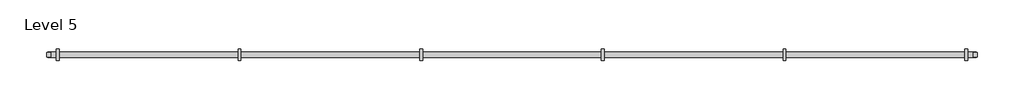
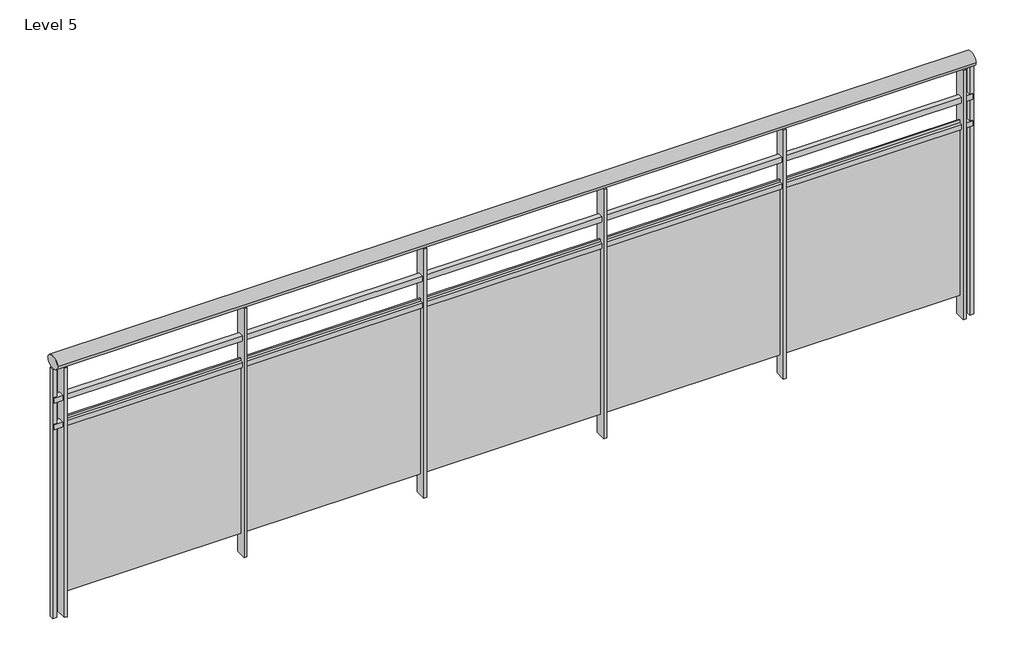
# One storey: 1 railing.
"""IFC4 building model written with IfcOpenShell, lengths in millimetres."""

from ifc_helpers import new_model, si_unit, point, frame, origin, place, context, project, spatial, polyline, ellipse_curve, trimmed, outline, extrude, element, save
from ifc_brep_helpers import plane_surface, extruded_surface, advanced_brep

model = new_model("IFC4")

# Units and contexts
model_context = context("Model", 3, world=origin())
ifc_project = project(units=[si_unit("LENGTHUNIT", "METRE", prefix="MILLI")], contexts=[model_context])

# Site, building, storey
site = spatial("IfcSite", under=ifc_project)
building = spatial("IfcBuilding", under=site)
storey = spatial("IfcBuildingStorey", under=building, Name="Level 5", Elevation=12801.6)

# Railing
placement = place(None, origin())
element("IfcRailing", 1, ObjectType="Glass Panel - Bottom Fill", at=placement, inside=storey, context=model_context, shape_type="SolidModel", body=[
    advanced_brep(
    [(-5729.1673724, -5829.5544725, 14020.8), (-5729.1673724, -5905.7544725, 14020.8), (-1576.8982041, -5829.5544725, 14020.8), (-1576.8982041, -5905.7544725, 14020.8)],
    [
        (0, 1, ellipse_curve(frame((-5729.1673724, -5867.6544725, 14020.8), z_axis=(-1.0, 0.0, 0.0), x_axis=(0.0, -1.0, 0.0)), 38.1, 28.575)),
        (1, 0, ellipse_curve(frame((-5729.1673724, -5867.6544725, 14020.8), z_axis=(-1.0, 0.0, 0.0), x_axis=(0.0, -1.0, 0.0)), 38.1, 28.575)),
        (2, 3, ellipse_curve(frame((-1576.8982041, -5867.6544725, 14020.8), z_axis=(1.0, 0.0, 0.0), x_axis=(0.0, -1.0, 0.0)), 38.1, 28.575)),
        (3, 2, ellipse_curve(frame((-1576.8982041, -5867.6544725, 14020.8), z_axis=(1.0, 0.0, 0.0), x_axis=(0.0, -1.0, 0.0)), 38.1, 28.575)),
        (0, 2),
        (3, 1),
    ],
    [
        plane_surface(frame((-5729.1673724, -5867.6544725, 14020.8), z_axis=(-1.0, 0.0, 0.0), x_axis=(0.0, 1.0, 0.0))),
        plane_surface(frame((-1576.8982041, -5867.6544725, 14020.8), z_axis=(1.0, 0.0, 0.0), x_axis=(0.0, 1.0, 0.0))),
        extruded_surface(trimmed(ellipse_curve(frame((-1576.8982041, -5867.6544725, 14020.8), z_axis=(-1.0, 0.0, 0.0), x_axis=(0.0, -1.0, 0.0)), 38.1, 28.575), [point((-1576.8982041, -5829.5544725, 14020.8))], [point((-1576.8982041, -5905.7544725, 14020.8))], True, "CARTESIAN"), (-4152.2691683, 0.0, 0.0), 4152.2691683),
        extruded_surface(trimmed(ellipse_curve(frame((-1576.8982041, -5867.6544725, 14020.8), z_axis=(-1.0, 0.0, 0.0), x_axis=(0.0, -1.0, 0.0)), 38.1, 28.575), [point((-1576.8982041, -5905.7544725, 14020.8))], [point((-1576.8982041, -5829.5544725, 14020.8))], True, "CARTESIAN"), (-4152.2691683, 0.0, 0.0), 4152.2691683),
    ],
    [
        (0, [[1, 2]]),
        (1, [[3, 4]]),
        (2, [[-1, 5, -4, 6]]),
        (3, [[-2, -6, -3, -5]]),
    ],
),
    extrude(outline(polyline([(-5729.1673724, -5880.3544725), (-5729.1673724, -5854.9544725), (-1576.8982041, -5854.9544725), (-1576.8982041, -5880.3544725), (-5729.1673724, -5880.3544725)])), frame((0.0, 0.0, 13830.3), z_axis=(0.0, 0.0, 1.0), x_axis=(1.0, 0.0, 0.0)), (0.0, 0.0, 1.0), 25.4),
    extrude(outline(polyline([(-5729.1673724, -5880.3544725), (-5729.1673724, -5854.9544725), (-1576.8982041, -5854.9544725), (-1576.8982041, -5880.3544725), (-5729.1673724, -5880.3544725)])), frame((0.0, 0.0, 13703.3), z_axis=(0.0, 0.0, 1.0), x_axis=(1.0, 0.0, 0.0)), (0.0, 0.0, 1.0), 25.4),
    extrude(outline(polyline([(-1627.3827882, -5893.0544725), (-1627.3827882, -5842.2544725), (-1614.6827882, -5842.2544725), (-1614.6827882, -5893.0544725), (-1627.3827882, -5893.0544725)])), frame((0.0, 0.0, 12801.6), z_axis=(0.0, 0.0, 1.0), x_axis=(1.0, 0.0, 0.0)), (0.0, 0.0, 1.0), 1190.625),
    extrude(outline(polyline([(-2433.8327882, -5861.1193155), (-1621.0327882, -5861.1193155), (-1621.0327882, -5867.4693155), (-2433.8327882, -5867.4693155), (-2433.8327882, -5861.1193155)])), frame((0.0, 0.0, 12903.2), z_axis=(0.0, 0.0, 1.0), x_axis=(1.0, 0.0, 0.0)), (0.0, 0.0, 1.0), 838.2),
    extrude(outline(polyline([(-2440.1827882, -5893.0544725), (-2440.1827882, -5842.2544725), (-2427.4827882, -5842.2544725), (-2427.4827882, -5893.0544725), (-2440.1827882, -5893.0544725)])), frame((0.0, 0.0, 12801.6), z_axis=(0.0, 0.0, 1.0), x_axis=(1.0, 0.0, 0.0)), (0.0, 0.0, 1.0), 1190.625),
    extrude(outline(polyline([(-3246.6327882, -5861.1193155), (-2433.8327882, -5861.1193155), (-2433.8327882, -5867.4693155), (-3246.6327882, -5867.4693155), (-3246.6327882, -5861.1193155)])), frame((0.0, 0.0, 12903.2), z_axis=(0.0, 0.0, 1.0), x_axis=(1.0, 0.0, 0.0)), (0.0, 0.0, 1.0), 838.2),
    extrude(outline(polyline([(-3252.9827882, -5893.0544725), (-3252.9827882, -5842.2544725), (-3240.2827882, -5842.2544725), (-3240.2827882, -5893.0544725), (-3252.9827882, -5893.0544725)])), frame((0.0, 0.0, 12801.6), z_axis=(0.0, 0.0, 1.0), x_axis=(1.0, 0.0, 0.0)), (0.0, 0.0, 1.0), 1190.625),
    extrude(outline(polyline([(-4059.4327882, -5861.1193155), (-3246.6327882, -5861.1193155), (-3246.6327882, -5867.4693155), (-4059.4327882, -5867.4693155), (-4059.4327882, -5861.1193155)])), frame((0.0, 0.0, 12903.2), z_axis=(0.0, 0.0, 1.0), x_axis=(1.0, 0.0, 0.0)), (0.0, 0.0, 1.0), 838.2),
    extrude(outline(polyline([(-4065.7827882, -5893.0544725), (-4065.7827882, -5842.2544725), (-4053.0827882, -5842.2544725), (-4053.0827882, -5893.0544725), (-4065.7827882, -5893.0544725)])), frame((0.0, 0.0, 12801.6), z_axis=(0.0, 0.0, 1.0), x_axis=(1.0, 0.0, 0.0)), (0.0, 0.0, 1.0), 1190.625),
    extrude(outline(polyline([(-4872.2327882, -5861.1193155), (-4059.4327882, -5861.1193155), (-4059.4327882, -5867.4693155), (-4872.2327882, -5867.4693155), (-4872.2327882, -5861.1193155)])), frame((0.0, 0.0, 12903.2), z_axis=(0.0, 0.0, 1.0), x_axis=(1.0, 0.0, 0.0)), (0.0, 0.0, 1.0), 838.2),
    extrude(outline(polyline([(-4878.5827882, -5893.0544725), (-4878.5827882, -5842.2544725), (-4865.8827882, -5842.2544725), (-4865.8827882, -5893.0544725), (-4878.5827882, -5893.0544725)])), frame((0.0, 0.0, 12801.6), z_axis=(0.0, 0.0, 1.0), x_axis=(1.0, 0.0, 0.0)), (0.0, 0.0, 1.0), 1190.625),
    extrude(outline(polyline([(-5685.0327882, -5861.1193155), (-4872.2327882, -5861.1193155), (-4872.2327882, -5867.4693155), (-5685.0327882, -5867.4693155), (-5685.0327882, -5861.1193155)])), frame((0.0, 0.0, 12903.2), z_axis=(0.0, 0.0, 1.0), x_axis=(1.0, 0.0, 0.0)), (0.0, 0.0, 1.0), 838.2),
    extrude(outline(polyline([(-5691.3827882, -5893.0544725), (-5691.3827882, -5842.2544725), (-5678.6827882, -5842.2544725), (-5678.6827882, -5893.0544725), (-5691.3827882, -5893.0544725)])), frame((0.0, 0.0, 12801.6), z_axis=(0.0, 0.0, 1.0), x_axis=(1.0, 0.0, 0.0)), (0.0, 0.0, 1.0), 1190.625),
    extrude(outline(polyline([(-1589.5982041, -5877.1794725), (-1589.5982041, -5858.1294725), (-1570.5482041, -5858.1294725), (-1570.5482041, -5877.1794725), (-1589.5982041, -5877.1794725)])), frame((0.0, 0.0, 12801.6), z_axis=(0.0, 0.0, 1.0), x_axis=(1.0, 0.0, 0.0)), (0.0, 0.0, 1.0), 1190.625),
    extrude(outline(polyline([(-5735.5173724, -5877.1794725), (-5735.5173724, -5858.1294725), (-5716.4673724, -5858.1294725), (-5716.4673724, -5877.1794725), (-5735.5173724, -5877.1794725)])), frame((0.0, 0.0, 12801.6), z_axis=(0.0, 0.0, 1.0), x_axis=(1.0, 0.0, 0.0)), (0.0, 0.0, 1.0), 1190.625),
])

save(model, "model.ifc")

# Revit data of these elements
# Type "Glass Panel - Bottom Fill"
#   Assembly Code = "C2010400"
#   built-in parameter 1008612 = 0.0416667 (stored number, unit not read)
#   built-in parameter 1008611 = 0.0416667 (stored number, unit not read)
#   built-in parameter 1008609 = 0.333333 (stored number, unit not read)
#   built-in parameter 1008604 = 0.166667 (stored number, unit not read)
#   built-in parameter 1008603 = 0.166667 (stored number, unit not read)
#   Railing Height = 4' - 0"
#   built-in parameter 1008630 = 2
#   built-in parameter 1008610 = 2
#   built-in parameter 1008618 = Baluster - Square : 3/4"
# Element 1 (IfcRailing, "Glass Panel - Bottom Fill")
#   Phase Created = New Construction
#   Materials on its faces: "Glass"
# Materials
#   "Glass": class "Glass", colour RGB 0 128 192, transparency 0.75, Description = "Soda Lime Glass", Cost = 0
